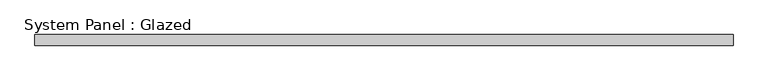
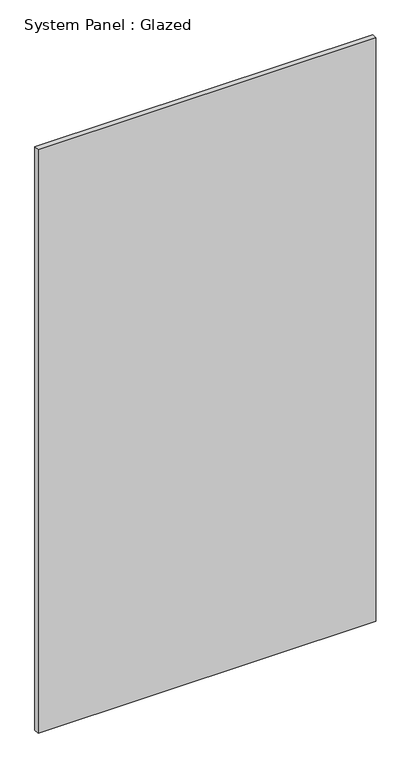
"""IFC4 building model written with IfcOpenShell, lengths in millimetres: plate geometry, System Panel : Glazed."""

from ifc_helpers import new_model, si_unit, origin, origin_with_axes, place, context, project, spatial, polyline, outline, extrude, source, transform, mapped, element, save


def system_panel_glazed_a38948d3(model_context):
    return source(origin(), model_context, "Body", "SweptSolid", [
        extrude(outline(polyline([(800.1, 19.05), (-800.1, 19.05), (-800.1, 44.45), (800.1, 44.45), (800.1, 19.05)])), origin_with_axes(), (0.0, 0.0, 1.0), 2921.0),
    ])


if __name__ == "__main__":
    model = new_model("IFC4")
    model_context = context("Model", 3, world=origin())
    ifc_project = project(units=[si_unit("LENGTHUNIT", "METRE", prefix="MILLI")], contexts=[model_context])
    site = spatial("IfcSite", under=ifc_project)
    building = spatial("IfcBuilding", under=site)
    placement = place(None, origin())
    system_panel_glazed_shape = system_panel_glazed_a38948d3(model_context)
    element("IfcPlate", 1, ObjectType="System Panel : Glazed", at=placement, inside=building, context=model_context, shape_type="MappedRepresentation", body=[
        mapped(system_panel_glazed_shape, transform((0.0, 0.0, 0.0), x_axis=(1.0, 0.0, 0.0), y_axis=(0.0, 1.0, 0.0), z_axis=(0.0, 0.0, 1.0))),
    ])
    save(model, "model.ifc")

# Revit data of these elements
# Type "System Panel : Glazed"
#   Construction Type Id = "GSP4R"
#   Analytic Construction = "1/8 in Pilkington single glazing"
#   Visual Light Transmittance = 0.9
#   Solar Heat Gain Coefficient = 0.86
#   Heat Transfer Coefficient (U) = 1.18115 BTU/(h·ft²·°F)
# Element 1 (IfcPlate, "System Panel : Glazed")
#   Materials on its faces: "Glass"
# Materials
#   "Glass": class "Glass", colour RGB 0 128 192, transparency 0.75, Description = "Soda Lime Glass", Cost = 0
